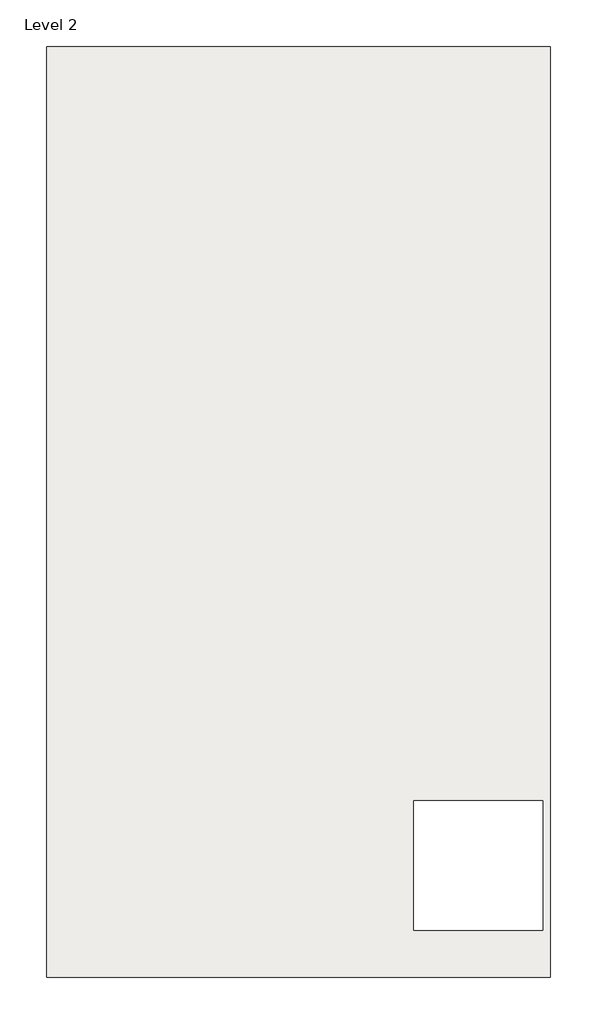
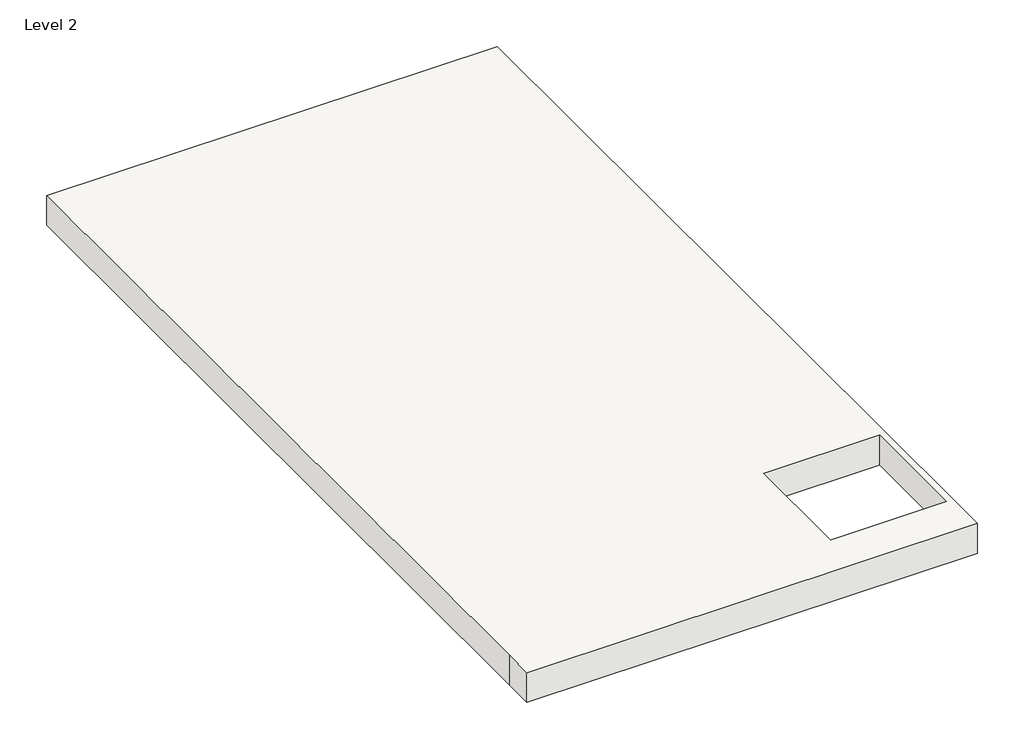
# One storey: 1 roof.
"""IFC4 building model written with IfcOpenShell, lengths in millimetres."""

from ifc_helpers import new_model, si_unit, frame, origin, place, context, project, spatial, polyline, outline, extrude, element, save

model = new_model("IFC4")

# Units and contexts
model_context = context("Model", 3, world=origin())
ifc_project = project(units=[si_unit("LENGTHUNIT", "METRE", prefix="MILLI")], contexts=[model_context])

# Site, building, storey
site = spatial("IfcSite", under=ifc_project)
building = spatial("IfcBuilding", under=site)
storey = spatial("IfcBuildingStorey", under=building, Name="Level 2", Elevation=3048.0)

# Roof
placement = place(None, origin())
element("IfcRoof", 1, ObjectType="Steel Truss - Insulation on Metal Deck - EPDM", at=placement, inside=storey, context=model_context, shape_type="SweptSolid", body=[
    extrude(outline(polyline([(-6217.3247449, 14665.2258877), (1605.8752551, 14665.2258877), (1605.8752551, 746.0258877), (1605.8752551, 212.6258877), (-6217.3247449, 212.6258877), (-6217.3247449, 746.0258877), (-6217.3247449, 14665.2258877)]), holes=[polyline([(1488.6340081, 2955.8258877), (-517.9659919, 2955.8258877), (-517.9659919, 1045.9647998), (-517.9659919, 949.2258877), (1488.6340081, 949.2258877), (1488.6340081, 2955.8258877)])]), frame((0.0, 0.0, 3048.0), z_axis=(0.0, 0.0, 1.0), x_axis=(1.0, 0.0, 0.0)), (0.0, 0.0, 1.0), 546.1),
])

save(model, "model.ifc")

# Revit data of these elements
# Type "Steel Truss - Insulation on Metal Deck - EPDM"
#   Assembly Code = "B1020"
#   Layers, outside or top first: 0' - 0 1/4" "Roofing, EPDM Membrane" (function 4); 0' - 5" "Rigid insulation" (function 3); 0' - 0 1/4" "Metal Deck" (function 1); 1' - 4" "Structure, Steel Bar Joist Layer" (function 1)
# Element 1 (IfcRoof, "Steel Truss - Insulation on Metal Deck - EPDM")
#   built-in parameter 1001705 = 11.7917 (stored number, unit not read)
#   built-in parameter 1001710 = 33615
#   Phase Created = New Construction
#   Materials on its faces: "Structure, Steel Bar Joist Layer", "Roofing, EPDM Membrane"
# Materials
#   "Roofing, EPDM Membrane": class "Generic", colour RGB 127 127 127, transparency 0, Description = "EPDM roof membrane", Cost = 0
#   "Rigid insulation": class "Generic", colour RGB 127 127 127, transparency 0, Description = "Rigid foam insulation board", Cost = 0
#   "Metal Deck": class "Metal", colour RGB 199 199 199, transparency 0, Description = "Steel, mill finish", Cost = 0
#   "Structure, Steel Bar Joist Layer": class "Metal", colour RGB 127 127 127, transparency 0, Description = "Bar joists, thermal airspace", Cost = 0
